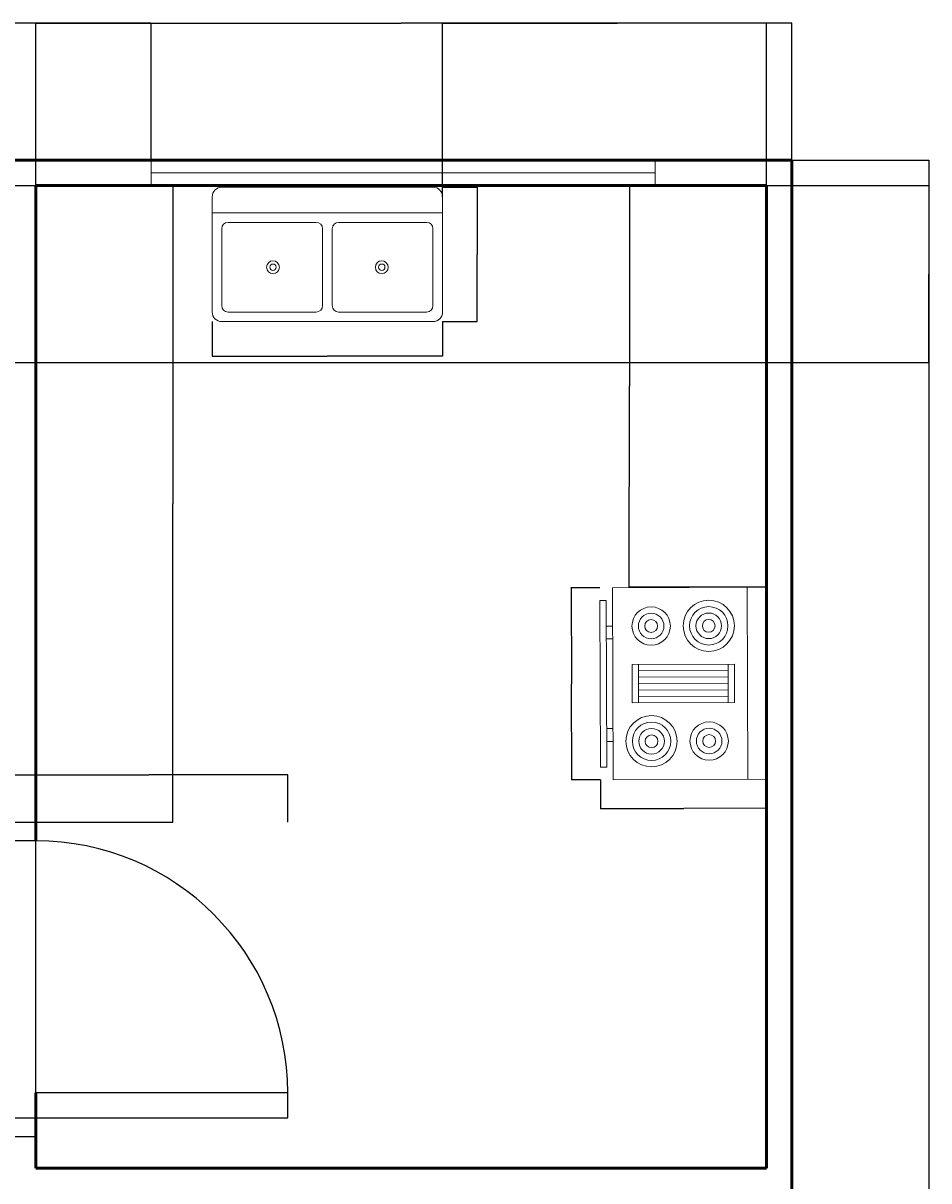
# Model space of a CAD drawing. Units: millimetres. Extents: x 1584 to 12772, y -932 to 10602.
# Tile 4 of 4: x 9178 to 12772, y 5860 to 10454. Entities that reach past the tile are written whole.
import ezdxf

# ---------------------------------------------------------------- set-up
doc = ezdxf.new("R2010")
doc.units = ezdxf.units.MM
for name, color, linetype, lineweight in [('A-ANNO-DIMS', 2, 'Continuous', 18), ('A-DOOR', 3, 'Continuous', 25), ('A-EQPM', 8, 'Continuous', 18), ('A-FLOR-FIXT', 9, 'Continuous', 18), ('A-GLAZ', 4, 'Continuous', 18), ('A-WALL', 7, 'Continuous', 50)]:
    doc.layers.add(name, color=color, linetype=linetype, lineweight=lineweight)
doc.styles.get("Standard").update_dxf_attribs({"font": 'arial.ttf'})
doc.dimstyles.get("Standard").update_dxf_attribs({"dimtxt": 0.18, "dimasz": 0.18, "dimexe": 0.18, "dimexo": 0.0625, "dimgap": 0.09, "dimtad": 0, "dimtih": 1, "dimtoh": 1, "dimdec": 4, "dimzin": 0, "dimdsep": 46, "dimtxsty": 'Standard', "dimcen": 0.09, "dimadec": 0, "dimazin": 0, "dimtfac": 1, "dimtdec": 4, "dimtofl": 0, "dimtmove": 0, "dimatfit": 3, "dimfxl": 1, "dimtolj": 1, "dimtzin": 0, "dimarcsym": 0})

# ---------------------------------------------------------------- blocks, each defined once
blk = doc.blocks.new('Range-Oven - 30 in top')
for p, q in [((0, -3), (30, -3)), ((12, -6), (18, -6)), ((13, -19.999996), (13, -6)), ((14, -6), (14, -19.999996)), ((15, -19.999996), (15, -6)), ((16, -6), (16, -19.999996)), ((17, -19.999996), (17, -6)), ((18, -19.999996), (12, -19.999996)), ((6.000000000000003, -23.99999600000001), (6.000000000000003, -24.999996)), ((8.000000000000004, -24.999996), (8.000000000000004, -23.99999600000001)), ((22.00000000000001, -24.999996), (22.00000000000001, -23.99999600000001)), ((24, -23.99999600000001), (24, -24.999996))]:
    blk.add_line(p, q)
for points in [[(0, -23.99999600000001), (0, 0), (30, 0), (30, -23.99999600000001)], [(12, -20.999996), (12, -5), (18, -5), (18, -20.999996)], [(2.000000000000003, -25.999996), (2.000000000000003, -24.999996), (28.00000000000001, -24.999996), (28.00000000000001, -25.999996)]]:
    blk.add_lwpolyline(points, close=True)
for centre, radius in [((6.000000000000003, -9.0000002), 4), ((6.000000000000003, -9.0000002), 3), ((6.000000000000003, -9.0000002), 2), ((24, -9.0000002), 3), ((24, -9.0000002), 2), ((6.000000000000003, -9.0000002), 1), ((24, -9.0000002), 1), ((24, -18), 4), ((6.000000000000003, -18), 3), ((6.000000000000003, -18), 2), ((24, -18), 3), ((24, -18), 2), ((6.000000000000003, -18), 1), ((24, -18), 1)]:
    blk.add_circle(centre, radius)
blk = doc.blocks.new('Sink-double - 36 in top')
for p, q in [((-18, -4), (18, -4)), ((-0.75, -18.5), (-0.75, -6.5)), ((0.75, -6.5), (0.75, -18.5))]:
    blk.add_line(p, q)
for points in [[(-16.5, 0), (16.5, 0)], [(-18, -19.5), (-18, -1.5)], [(18, -1.5), (18, -19.5)], [(-16.5, -18.5), (-16.5, -6.5)], [(-15.5, -5.5), (-1.75, -5.5)], [(1.75, -5.5), (15.5, -5.5)], [(16.5, -6.5), (16.5, -18.5)], [(-1.75, -19.5), (-15.5, -19.5)], [(15.5, -19.5), (1.75, -19.5)], [(16.5, -21), (-16.5, -21)]]:
    blk.add_lwpolyline(points)
for centre, radius in [((-8.5, -12.5), 1), ((-8.5, -12.5), 0.5), ((8.5, -12.5), 1), ((8.5, -12.5), 0.5)]:
    blk.add_circle(centre, radius)
for centre, radius, start, end in [((-16.5, -1.5), 1.5, 90, 180), ((16.5, -1.5), 1.5, 0, 90), ((-15.5, -6.5), 1, 90, 180), ((-1.75, -6.5), 1, 0, 90), ((1.75, -6.5), 1, 90, 180), ((15.5, -6.5), 1, 0, 90), ((-16.5, -19.5), 1.5, 180, 270), ((-15.5, -18.5), 1, 180, 270), ((-1.75, -18.5), 1, 270, 0), ((1.75, -18.5), 1, 180, 270), ((15.5, -18.5), 1, 270, 0), ((16.5, -19.5), 1.5, 270, 0)]:
    blk.add_arc(centre, radius, start, end)
blk = doc.blocks.new('DOOR-SINGLE-1000')
for p, q in [((1000.000230036349, 1174.20008536707), (1000.000230036349, 1248.400085367071)), ((1000.000230036349, 1248.400085367071), (1100.000230036349, 1248.400085367071)), ((1100.000230036349, 1248.400085367071), (1100.000230036349, 1174.20008536707)), ((1000.000230036349, 1174.20008536707), (0.0002300363494214, 1174.20008536707)), ((0.0002300363494214, 1174.20008536707), (0.0002300363494214, 1074.200085367071)), ((1000.000230036349, 1074.200085367071), (1000.000230036349, 1174.20008536707)), ((1100.000230036349, 1174.20008536707), (1000.000230036349, 1174.20008536707)), ((0.0002300363494214, 1074.200085367071), (1000.000230036349, 1074.200085367071)), ((1000.000230036349, 8.53670690049e-05), (1000.000230036349, 74.20008536706973)), ((1000.000230036349, 74.20008536706973), (1100.000230036349, 74.20008536706973)), ((1100.000230036349, 74.20008536706973), (1100.000230036349, 8.53670690049e-05)), ((1100.000230036349, 8.53670690049e-05), (1000.000230036349, 8.53670690049e-05))]:
    blk.add_line(p, q)
blk.add_arc((1000.000230036349, 1074.200085367071), 1000.000000000001, 180, 270)
blk = doc.blocks.new('WIN-2000')
for p, q in [((-0.0004293290949136, 99.99960647437545), (1999.999570670905, 99.99960647437545)), ((-0.0004293290949136, -0.0003935256245313), (-0.0004293290949136, 99.99960647437545)), ((1999.999570670905, 99.99960647437545), (1999.999570670905, -0.0003935256245313)), ((-0.0004293290949136, 49.99960647437365), (1999.999570670905, 49.99960647437183)), ((1999.999570670905, -0.0003935256245313), (-0.0004293290949136, -0.0003935256245313))]:
    blk.add_line(p, q)
blk = doc.blocks.new('*D13')
at = {"layer": 'A-ANNO-DIMS', "color": 0, "lineweight": -2, "transparency": 16777216}
for p, q in [((9127.833230036342, 7283.882915011043), (9127.833230036342, 7471.260415011044)), ((9128.013230036344, 7471.080415011043), (9677.173762096369, 7471.080415011043)), ((10227.65323003634, 7471.080415011043), (9678.492697976317, 7471.080415011043)), ((10227.83323003634, 7283.882915011043), (10227.83323003634, 7471.260415011044))]:
    blk.add_line(p, q, dxfattribs=at)
at = {"layer": 'A-ANNO-DIMS', "color": 0, "transparency": 16777216}
for points in [[(9128.013230036344, 7471.110415011043), (9128.013230036344, 7471.050415011044), (9127.833230036342, 7471.080415011043)], [(10227.65323003634, 7471.110415011043), (10227.65323003634, 7471.050415011044), (10227.83323003634, 7471.080415011043)]]:
    blk.add_solid(points, dxfattribs=at)
at = {"layer": 'Defpoints', "color": 0, "transparency": 16777216}
for p in [(9127.833230036342, 7471.080415011043), (9127.833230036342, 7283.820415011042), (10227.83323003634, 7283.820415011042)]:
    blk.add_point(p, dxfattribs=at)
at = {"layer": 'A-ANNO-DIMS', "color": 0, "transparency": 16777216, "insert": (9677.833230036342, 7471.080415011043), "char_height": 0.18, "attachment_point": 5}
blk.add_mtext('\\A1;1100 TYP.', dxfattribs=at)
blk = doc.blocks.new('*D24')
at = {"layer": 'A-ANNO-DIMS', "color": 0, "lineweight": -2, "transparency": 16777216}
for p, q in [((11466.12116221621, 8213.449737593239), (11351.70437339575, 8213.046324324887)), ((11351.88500692101, 8212.866960087778), (11353.22705676214, 7832.232396710056)), ((11354.57039754488, 7451.231694178173), (11353.22834770374, 7831.866257555894)), ((11468.80782212823, 7451.454473921266), (11354.39103330777, 7451.051060652917))]:
    blk.add_line(p, q, dxfattribs=at)
at = {"layer": 'A-ANNO-DIMS', "color": 0, "transparency": 16777216}
for points in [[(11351.91500673454, 8212.86706586179), (11351.85500710748, 8212.866854313766), (11351.88437227693, 8213.046958968964)], [(11354.60039735841, 7451.231799952186), (11354.54039773135, 7451.231588404161), (11354.57103218895, 7451.051695296991)]]:
    blk.add_solid(points, dxfattribs=at)
at = {"layer": 'Defpoints', "color": 0, "transparency": 16777216}
for p in [(11466.18366182773, 8213.449957955765), (11354.57103218895, 7451.051695296991), (11468.87032173975, 7451.454694283794)]:
    blk.add_point(p, dxfattribs=at)
at = {"layer": 'A-ANNO-DIMS', "color": 0, "transparency": 16777216, "insert": (11353.22770223294, 7832.049327132977), "char_height": 0.18, "attachment_point": 5}
blk.add_mtext('\\A1;RANGE 762', dxfattribs=at)
blk = doc.blocks.new('*D25')
at = {"layer": 'A-ANNO-DIMS', "color": 0, "lineweight": -2, "transparency": 16777216}
for p, q in [((11468.87054210228, 7451.392194672272), (11469.27395537063, 7336.975405851815)), ((12129.26633568528, 7453.720632904467), (12129.66974895363, 7339.30384408401)), ((11469.45331960773, 7337.156039377072), (11799.18218614015, 7338.31860477581)), ((12129.48911542837, 7339.483208321119), (11799.76024889595, 7338.32064292238))]:
    blk.add_line(p, q, dxfattribs=at)
at = {"layer": 'A-ANNO-DIMS', "color": 0, "transparency": 16777216}
for points in [[(11469.45321383372, 7337.186039190602), (11469.45342538175, 7337.126039563542), (11469.27332072655, 7337.155404732998)], [(12129.48900965436, 7339.513208134649), (12129.48922120239, 7339.453208507589), (12129.66911430956, 7339.483842965193)]]:
    blk.add_solid(points, dxfattribs=at)
at = {"layer": 'Defpoints', "color": 0, "transparency": 16777216}
for p in [(11468.87032173975, 7451.454694283794), (12129.26611532276, 7453.783132515988), (12129.66911430956, 7339.483842965193)]:
    blk.add_point(p, dxfattribs=at)
at = {"layer": 'A-ANNO-DIMS', "color": 0, "transparency": 16777216, "insert": (11799.47121751805, 7338.319623849095), "char_height": 0.18, "attachment_point": 5}
blk.add_mtext('\\A1;660', dxfattribs=at)
blk = doc.blocks.new('*D26')
at = {"layer": 'A-ANNO-DIMS', "color": 0, "lineweight": -2, "transparency": 16777216}
for p, q in [((9927.831256270129, 9269.57878250212), (9927.831256270129, 9132.301282502123)), ((10842.23125627013, 9269.57878250212), (10842.23125627013, 9132.301282502123)), ((9928.01125627013, 9132.481282502124), (10383.86690429196, 9132.481282502124)), ((10842.05125627013, 9132.481282502124), (10386.1956082483, 9132.481282502124))]:
    blk.add_line(p, q, dxfattribs=at)
at = {"layer": 'A-ANNO-DIMS', "color": 0, "transparency": 16777216}
for points in [[(9928.01125627013, 9132.511282502122), (9928.01125627013, 9132.451282502121), (9927.831256270129, 9132.481282502124)], [(10842.05125627013, 9132.511282502122), (10842.05125627013, 9132.451282502121), (10842.23125627013, 9132.481282502124)]]:
    blk.add_solid(points, dxfattribs=at)
at = {"layer": 'Defpoints', "color": 0, "transparency": 16777216}
for p in [(9927.831256270129, 9269.641282502122), (10842.23125627013, 9269.641282502122), (10842.23125627013, 9132.481282502124)]:
    blk.add_point(p, dxfattribs=at)
at = {"layer": 'A-ANNO-DIMS', "color": 0, "transparency": 16777216, "insert": (10385.03125627013, 9132.481282502124), "char_height": 0.18, "attachment_point": 5}
blk.add_mtext('\\A1;DOUBLE SINK 914', dxfattribs=at)
blk = doc.blocks.new('*D27')
at = {"layer": 'A-ANNO-DIMS', "color": 0, "lineweight": -2, "transparency": 16777216}
for p, q in [((10842.29375627013, 9803.041282502123), (10979.57125627013, 9803.041282502123)), ((10979.39125627013, 9802.861282502123), (10979.39125627013, 9536.523247031455)), ((10979.39125627013, 9269.821282502126), (10979.39125627013, 9536.159317972793)), ((10842.29375627013, 9269.641282502125), (10979.57125627013, 9269.641282502125))]:
    blk.add_line(p, q, dxfattribs=at)
at = {"layer": 'A-ANNO-DIMS', "color": 0, "transparency": 16777216}
for points in [[(10979.36125627013, 9802.861282502123), (10979.42125627014, 9802.861282502123), (10979.39125627013, 9803.041282502123)], [(10979.36125627013, 9269.821282502126), (10979.42125627014, 9269.821282502126), (10979.39125627013, 9269.641282502125)]]:
    blk.add_solid(points, dxfattribs=at)
at = {"layer": 'Defpoints', "color": 0, "transparency": 16777216}
for p in [(10842.23125627013, 9803.041282502123), (10979.39125627013, 9803.041282502123), (10842.23125627013, 9269.641282502125)]:
    blk.add_point(p, dxfattribs=at)
at = {"layer": 'A-ANNO-DIMS', "color": 0, "transparency": 16777216, "insert": (10979.39125627013, 9536.341282502119), "char_height": 0.18, "attachment_point": 5}
blk.add_mtext('\\A1;533', dxfattribs=at)
blk = doc.blocks.new('*D37')
at = {"layer": 'A-ANNO-DIMS', "color": 0, "lineweight": -2, "transparency": 16777216}
for p, q in [((12227.89573, 9910.180606000004), (12771.71323000001, 9910.180606000005)), ((12771.53323000001, 9910.000606000005), (12771.53323000001, 4761.453150137792)), ((12771.53323000001, -387.4581119999995), (12771.53323000001, 4761.089343862212)), ((8227.895730000006, -387.6381120000002), (12771.71323000001, -387.6381119999995))]:
    blk.add_line(p, q, dxfattribs=at)
at = {"layer": 'A-ANNO-DIMS', "color": 0, "transparency": 16777216}
for points in [[(12771.50323000001, 9910.000606000005), (12771.56323000001, 9910.000606000005), (12771.53323000001, 9910.180606000005)], [(12771.50323000001, -387.4581119999995), (12771.56323000001, -387.4581119999995), (12771.53323000001, -387.6381119999995)]]:
    blk.add_solid(points, dxfattribs=at)
at = {"layer": 'Defpoints', "color": 0, "transparency": 16777216}
for p in [(12227.83323, 9910.180606000004), (12771.53323000001, 9910.180606000005), (8227.833230000006, -387.6381120000002)]:
    blk.add_point(p, dxfattribs=at)
at = {"layer": 'A-ANNO-DIMS', "color": 0, "transparency": 16777216, "insert": (12771.53323000001, 4761.271246999998), "char_height": 0.18, "attachment_point": 5}
blk.add_mtext('\\A1;10298', dxfattribs=at)
blk = doc.blocks.new('*D45')
at = {"layer": 'A-ANNO-DIMS', "color": 0, "lineweight": -2, "transparency": 16777216}
for p, q in [((9227.833229999998, 5910.243106), (9227.833229999998, 10454.060606)), ((9228.01323, 10453.880606), (10677.47323, 10453.880606)), ((12127.65323, 10453.880606), (10678.19323, 10453.880606)), ((12127.83323, 5910.243106), (12127.83323, 10454.060606))]:
    blk.add_line(p, q, dxfattribs=at)
at = {"layer": 'A-ANNO-DIMS', "color": 0, "transparency": 16777216}
for points in [[(9228.01323, 10453.910606), (9228.01323, 10453.850606), (9227.833229999998, 10453.880606)], [(12127.65323, 10453.910606), (12127.65323, 10453.850606), (12127.83323, 10453.880606)]]:
    blk.add_solid(points, dxfattribs=at)
at = {"layer": 'Defpoints', "color": 0, "transparency": 16777216}
for p in [(12127.83323, 10453.880606), (9227.833229999998, 5910.180606), (12127.83323, 5910.180606)]:
    blk.add_point(p, dxfattribs=at)
at = {"layer": 'A-ANNO-DIMS', "color": 0, "transparency": 16777216, "insert": (10677.83323, 10453.880606), "char_height": 0.18, "attachment_point": 5}
blk.add_mtext('\\A1;2900', dxfattribs=at)
blk = doc.blocks.new('*D53')
at = {"layer": 'A-ANNO-DIMS', "color": 0, "lineweight": -2, "transparency": 16777216}
for p, q in [((8177.781093, 9910.243106000002), (8177.781093, 10454.060606)), ((8177.961093, 10453.880606), (8931.027043459755, 10453.880606)), ((9685.002571, 10453.880606), (8931.936620540248, 10453.880606)), ((9685.182571, 9910.243106000002), (9685.182571, 10454.060606))]:
    blk.add_line(p, q, dxfattribs=at)
at = {"layer": 'A-ANNO-DIMS', "color": 0, "transparency": 16777216}
for points in [[(8177.961093, 10453.910606), (8177.961093, 10453.850606), (8177.781093, 10453.880606)], [(9685.002571, 10453.910606), (9685.002571, 10453.850606), (9685.182571, 10453.880606)]]:
    blk.add_solid(points, dxfattribs=at)
at = {"layer": 'Defpoints', "color": 0, "transparency": 16777216}
for p in [(9685.182571, 10453.880606), (8177.781093, 9910.180606), (9685.182571, 9910.180606)]:
    blk.add_point(p, dxfattribs=at)
at = {"layer": 'A-ANNO-DIMS', "color": 0, "transparency": 16777216, "insert": (8931.481832000001, 10453.880606), "char_height": 0.18, "attachment_point": 5}
blk.add_mtext('\\A1;1507.4', dxfattribs=at)
blk = doc.blocks.new('*D58')
at = {"layer": 'A-ANNO-DIMS', "color": 0, "lineweight": -2, "transparency": 16777216}
for p, q in [((9227.895730000006, 9810.180606000004), (9771.713230000008, 9810.180606000004)), ((9771.533230000008, 9810.000606000003), (9771.533230000008, 8547.182413637793)), ((9771.533230000008, 7284.000415000004), (9771.533230000008, 8546.818607362215)), ((9227.895730000006, 7283.820415000004), (9771.713230000008, 7283.820415000004))]:
    blk.add_line(p, q, dxfattribs=at)
at = {"layer": 'A-ANNO-DIMS', "color": 0, "transparency": 16777216}
for points in [[(9771.503230000008, 9810.000606000003), (9771.563230000007, 9810.000606000003), (9771.533230000008, 9810.180606000004)], [(9771.503230000008, 7284.000415000004), (9771.563230000007, 7284.000415000004), (9771.533230000008, 7283.820415000004)]]:
    blk.add_solid(points, dxfattribs=at)
at = {"layer": 'Defpoints', "color": 0, "transparency": 16777216}
for p in [(9227.833230000006, 9810.180606000004), (9227.833230000006, 7283.820415000004), (9771.533230000008, 7283.820415000004)]:
    blk.add_point(p, dxfattribs=at)
at = {"layer": 'A-ANNO-DIMS', "color": 0, "transparency": 16777216, "insert": (9771.533230000008, 8547.0005105), "char_height": 0.18, "attachment_point": 5}
blk.add_mtext('\\A1;2526.4', dxfattribs=at)
blk = doc.blocks.new('*D67')
at = {"layer": 'A-ANNO-DIMS', "color": 0, "lineweight": -2, "transparency": 16777216}
for p, q in [((11584.13325676786, 9810.428150027006), (11583.50665404139, 9013.588948109002)), ((12127.77073001932, 9810.18065514751), (11583.95339836833, 9810.60829151617)), ((11582.8797652321, 8216.385939915408), (11583.50636795857, 9013.225141833422)), ((12126.51695501932, 8215.77844514751), (11582.69962374294, 8216.206081515877))]:
    blk.add_line(p, q, dxfattribs=at)
at = {"layer": 'A-ANNO-DIMS', "color": 0, "transparency": 16777216}
for points in [[(11584.10325677714, 9810.42817361781), (11584.16325675859, 9810.428126436207), (11584.13339831267, 9810.608149971358)], [(11582.84976524138, 8216.38596350621), (11582.90976522283, 8216.385916324605), (11582.87962368729, 8216.205939971062)]]:
    blk.add_solid(points, dxfattribs=at)
at = {"layer": 'Defpoints', "color": 0, "transparency": 16777216}
for p in [(11584.13339831267, 9810.608149971358), (12127.83323, 9810.180606000004), (12126.579455, 8215.778396000002)]:
    blk.add_point(p, dxfattribs=at)
at = {"layer": 'A-ANNO-DIMS', "color": 0, "transparency": 16777216, "insert": (11583.50651099998, 9013.407044971205), "char_height": 0.18, "attachment_point": 5}
blk.add_mtext('\\A1;1594.4', dxfattribs=at)
blk = doc.blocks.new('*D68')
at = {"layer": 'A-ANNO-DIMS', "color": 0, "lineweight": -2, "transparency": 16777216}
for p, q in [((10842.231256, 9765.003783), (10842.231256, 10454.060606)), ((10842.411256, 10453.880606), (11534.57714750204, 10453.880606)), ((12227.65323, 10453.880606), (11535.48733849795, 10453.880606)), ((12227.83323, 9910.243106000002), (12227.83323, 10454.060606))]:
    blk.add_line(p, q, dxfattribs=at)
at = {"layer": 'A-ANNO-DIMS', "color": 0, "transparency": 16777216}
for points in [[(10842.411256, 10453.910606), (10842.411256, 10453.850606), (10842.231256, 10453.880606)], [(12227.65323, 10453.910606), (12227.65323, 10453.850606), (12227.83323, 10453.880606)]]:
    blk.add_solid(points, dxfattribs=at)
at = {"layer": 'Defpoints', "color": 0, "transparency": 16777216}
for p in [(12227.83323, 10453.880606), (12227.83323, 9910.180606), (10842.231256, 9764.941283)]:
    blk.add_point(p, dxfattribs=at)
at = {"layer": 'A-ANNO-DIMS', "color": 0, "transparency": 16777216, "insert": (11535.032243, 10453.880606), "char_height": 0.18, "attachment_point": 5}
blk.add_mtext('\\A1;1385.6', dxfattribs=at)
blk = doc.blocks.new('*D75')
at = {"layer": 'A-ANNO-DIMS', "color": 0, "lineweight": -2, "transparency": 16777216}
for p, q in [((5227.895730000002, 9810.180606000004), (12771.71323000001, 9810.180606000005)), ((12771.53323000001, 9810.000606000007), (12771.53323000001, 9458.68676102934)), ((12771.53323000001, 9107.008987000005), (12771.53323000001, 9458.322831970676)), ((5551.087991000002, 9106.828987000004), (12771.71323000001, 9106.828987000004))]:
    blk.add_line(p, q, dxfattribs=at)
at = {"layer": 'A-ANNO-DIMS', "color": 0, "transparency": 16777216}
for points in [[(12771.50323000001, 9810.000606000007), (12771.56323000001, 9810.000606000007), (12771.53323000001, 9810.180606000005)], [(12771.50323000001, 9107.008987000005), (12771.56323000001, 9107.008987000005), (12771.53323000001, 9106.828987000004)]]:
    blk.add_solid(points, dxfattribs=at)
at = {"layer": 'Defpoints', "color": 0, "transparency": 16777216}
for p in [(5227.833230000002, 9810.180606000004), (5551.025491000002, 9106.828987000004), (12771.53323000001, 9106.828987000004)]:
    blk.add_point(p, dxfattribs=at)
at = {"layer": 'A-ANNO-DIMS', "color": 0, "transparency": 16777216, "insert": (12771.53323000001, 9458.504796500001), "char_height": 0.18, "attachment_point": 5}
blk.add_mtext('\\A1;703.4', dxfattribs=at)

msp = doc.modelspace()

# ---------------------------------------------------------------- linework, layer by layer
at = {"layer": 'A-GLAZ'}
msp.add_line((11685.1825706709, 9860.180606474376), (9685.182570670908, 9860.180606474376), dxfattribs=at)
msp.add_line((11685.1825706709, 9860.180606474376), (9685.182570670908, 9860.180606474376), dxfattribs=at)
at = {"layer": 'A-WALL'}
for p, q in [((2127.833230036349, 9910.180606474376), (12227.83323003635, 9910.180606474376)), ((12227.83323003635, 9910.180606474378), (12227.83323003635, 810.1806064743769)), ((9227.83323003635, 9810.18060647438), (9227.83323003635, 7209.620415011039)), ((9227.833230036349, 9810.18060647438), (12127.83323003635, 9810.180606474374)), ((12127.83323003635, 9810.180606474374), (12127.83323003635, 5910.180606474376)), ((9227.83323003635, 6209.620415011039), (9227.83323003635, 5910.180606474376)), ((9227.833230036349, 5910.180606474376), (12127.83323003635, 5910.180606474376))]:
    msp.add_line(p, q, dxfattribs=at)

# ---------------------------------------------------------------- block references
at = {"layer": 'A-DOOR', "rotation": 180}
msp.add_blockref('DOOR-SINGLE-1000', (10227.83346007269, 7283.820500378111), dxfattribs=at)
at = {"layer": 'A-EQPM', "xscale": 25.4, "yscale": 25.4, "zscale": 25.4, "rotation": 270.202013901418}
msp.add_blockref('Range-Oven - 30 in top', (12126.57945541074, 8215.778396187961), dxfattribs=at)
at = {"layer": 'A-FLOR-FIXT', "xscale": 25.4, "yscale": 25.4, "zscale": 25.4}
msp.add_blockref('Sink-double - 36 in top', (10385.03125627013, 9803.041282502121), dxfattribs=at)
at = {"layer": 'A-GLAZ'}
msp.add_blockref('WIN-2000', (9685.183000000003, 9810.181), dxfattribs=at)

# ---------------------------------------------------------------- dimensions: what is measured, and where the dimension line sits
at = {"layer": 'A-ANNO-DIMS'}
for base, p1, p2, override, picture, middle in [((9685.182571, 10453.880606), (8177.781093, 9910.180606), (9685.182571, 9910.180606), {"dimdec": 1, "dimlfac": 1, "dimrnd": 0, "dimzin": 0, "dimdsep": 46, "dimlunit": 2}, '*D53', (8931.481832000001, 10453.880606)), ((12127.83323, 10453.880606), (9227.833229999998, 5910.180606), (12127.83323, 5910.180606), {"dimdec": 0, "dimlfac": 1, "dimrnd": 0, "dimzin": 0, "dimdsep": 46, "dimlunit": 2}, '*D45', (10677.83323, 10453.880606)), ((12227.83323, 10453.880606), (10842.231256, 9764.941283), (12227.83323, 9910.180606), {"dimdec": 1, "dimlfac": 1, "dimrnd": 0, "dimzin": 0, "dimdsep": 46, "dimlunit": 2}, '*D68', (11535.032243, 10453.880606))]:
    dim = msp.add_linear_dim(base=base, p1=p1, p2=p2, dimstyle='Standard', override=override, dxfattribs=at)
    dim.commit()
    dim.dimension.update_dxf_attribs({"geometry": picture, "text_midpoint": middle})
for base, p1, p2, angle, override, picture, middle in [((12771.53323000001, 9910.180606000005), (8227.833229999998, -387.638112), (12227.83323, 9910.180606), 90, {"dimdec": 0, "dimlfac": 1, "dimrnd": 0, "dimzin": 0, "dimdsep": 46, "dimlunit": 2}, '*D37', (12771.53323000001, 4761.271246999998)), ((12771.53323000001, 9106.828987000004), (5227.83323, 9810.180606000002), (5551.025491, 9106.828987), 90, {"dimdec": 1, "dimlfac": 1, "dimrnd": 0, "dimzin": 0, "dimdsep": 46, "dimlunit": 2}, '*D75', (12771.53323000001, 9458.504796500001)), ((9771.533230000008, 7283.820415000004), (9227.833229999998, 9810.180606000002), (9227.833229999998, 7283.820415), 269.9999999999998, {"dimdec": 1, "dimlfac": 1, "dimrnd": 0, "dimzin": 0, "dimdsep": 46, "dimlunit": 2}, '*D58', (9771.533230000008, 8547.0005105)), ((10979.39125627013, 9803.041282502123), (10842.23125627013, 9269.641282502122), (10842.23125627013, 9803.041282502121), 90, {"dimdec": 0, "dimlfac": 1, "dimrnd": 0, "dimzin": 0, "dimdsep": 46, "dimlunit": 2}, '*D27', (10979.39125627013, 9536.341282502119)), ((11584.13339831267, 9810.608149971358), (12126.579455, 8215.778396000002), (12127.83323, 9810.180606000002), 89.95494488201423, {"dimdec": 1, "dimlfac": 1, "dimrnd": 0, "dimzin": 0, "dimdsep": 46, "dimlunit": 2}, '*D67', (11583.50651099998, 9013.407044971205)), ((12129.66911430956, 7339.483842965193), (11468.87032173975, 7451.454694283794), (12129.26611532276, 7453.78313251599), 0.2020139014180131, {"dimdec": 0, "dimlfac": 1, "dimrnd": 0, "dimzin": 0, "dimdsep": 46, "dimlunit": 2}, '*D25', (11799.47121751805, 7338.319623849095))]:
    dim = msp.add_linear_dim(base=base, p1=p1, p2=p2, angle=angle, dimstyle='Standard', override=override, dxfattribs=at)
    dim.commit()
    dim.dimension.update_dxf_attribs({"geometry": picture, "text_midpoint": middle})
dim = msp.add_linear_dim(base=(10842.23125627013, 9132.481282502124), p1=(9927.831256270129, 9269.641282502122), p2=(10842.23125627013, 9269.641282502122), text='DOUBLE SINK <>', dimstyle='Standard', override={"dimdec": 0, "dimlfac": 1, "dimrnd": 0, "dimzin": 0, "dimdsep": 46, "dimlunit": 2}, dxfattribs=at)
dim.commit()
dim.dimension.update_dxf_attribs({"geometry": '*D26', "text_midpoint": (10385.03125627013, 9132.481282502124)})
for base, p1, p2, angle, text, picture, middle in [((11354.57103218895, 7451.051695296991), (11466.18366182773, 8213.449957955765), (11468.87032173975, 7451.454694283794), 270.202013901418, 'RANGE <>', '*D24', (11353.22770223294, 7832.049327132977)), ((9127.833230036342, 7471.080415011043), (10227.83323003634, 7283.820415011042), (9127.833230036342, 7283.820415011042), 180, '<> TYP.', '*D13', (9677.833230036342, 7471.080415011043))]:
    dim = msp.add_linear_dim(base=base, p1=p1, p2=p2, angle=angle, text=text, dimstyle='Standard', override={"dimdec": 0, "dimlfac": 1, "dimrnd": 0, "dimzin": 0, "dimdsep": 46, "dimlunit": 2}, dxfattribs=at)
    dim.commit()
    dim.dimension.update_dxf_attribs({"geometry": picture, "text_midpoint": middle})

doc.saveas('drawing.dxf')
